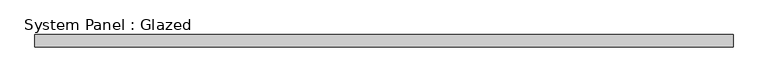
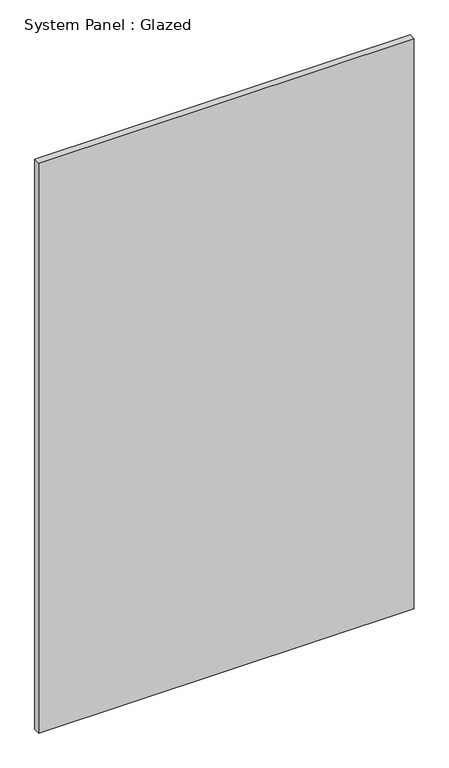
"""IFC4 building model written with IfcOpenShell, lengths in millimetres: plate geometry, System Panel : Glazed."""

from ifc_helpers import new_model, si_unit, origin, origin_with_axes, place, context, project, spatial, polyline, outline, extrude, source, transform, mapped, element, save


def system_panel_glazed_d986c6a7(model_context):
    return source(origin(), model_context, "Body", "SweptSolid", [
        extrude(outline(polyline([(730.2499999, 19.05), (-730.2499999, 19.05), (-730.2499999, 44.45), (730.2499999, 44.45), (730.2499999, 19.05)])), origin_with_axes(), (0.0, 0.0, 1.0), 2343.15),
    ])


if __name__ == "__main__":
    model = new_model("IFC4")
    model_context = context("Model", 3, world=origin())
    ifc_project = project(units=[si_unit("LENGTHUNIT", "METRE", prefix="MILLI")], contexts=[model_context])
    site = spatial("IfcSite", under=ifc_project)
    building = spatial("IfcBuilding", under=site)
    placement = place(None, origin())
    system_panel_glazed_shape = system_panel_glazed_d986c6a7(model_context)
    element("IfcPlate", 1, ObjectType="System Panel : Glazed", at=placement, inside=building, context=model_context, shape_type="MappedRepresentation", body=[
        mapped(system_panel_glazed_shape, transform((0.0, 0.0, 0.0), x_axis=(1.0, 0.0, 0.0), y_axis=(0.0, 1.0, 0.0), z_axis=(0.0, 0.0, 1.0))),
    ])
    save(model, "model.ifc")

# Revit data of these elements
# Type "System Panel : Glazed"
#   Construction Type Id = "GSP4R"
#   Analytic Construction = "1/8 in Pilkington single glazing"
#   Visual Light Transmittance = 0.9
#   Solar Heat Gain Coefficient = 0.86
#   Heat Transfer Coefficient (U) = 1.18115 BTU/(h·ft²·°F)
#   Define Thermal Properties by = 1
# Element 1 (IfcPlate, "System Panel : Glazed")
#   Materials on its faces: "Glass"
# Materials
#   "Glass": class "Glass", colour RGB 0 128 192, transparency 0.75, Description = "Soda Lime Glass", Cost = 0
